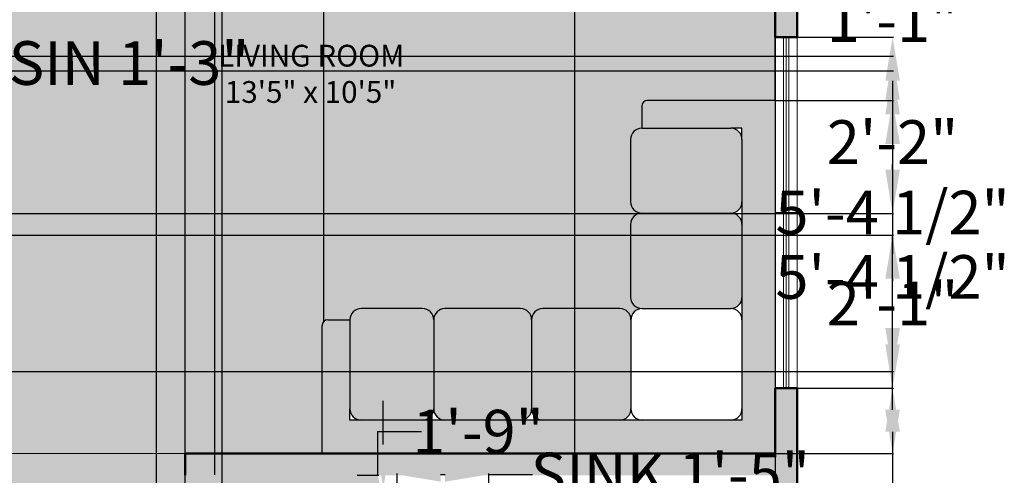
# Model space of a CAD drawing. Units: inches. Extents: x 339 to 824, y 73 to 445.
# Tile 4 of 5: x 605 to 785, y 213 to 297. Entities that reach past the tile are written whole.
import ezdxf

# ---------------------------------------------------------------- set-up
doc = ezdxf.new("R2010")
doc.units = ezdxf.units.IN
doc.header["$MEASUREMENT"] = 0
for name, color, linetype, lineweight in [('A-ANNO-DIMS', 2, 'Continuous', 18), ('A-AREA-IDEN', 7, 'Continuous', 25), ('A-DOOR', 3, 'Continuous', 25), ('A-FLOR-BNDY', 8, 'Continuous', 13), ('A-FLOR-PATT', 8, 'Continuous', 13), ('A-FURN', 9, 'Continuous', 25), ('A-GLAZ', 4, 'Continuous', 18), ('A-WALL', 7, 'Continuous', 50), ('A-WALL-PATT', 1, 'Continuous', 13)]:
    doc.layers.add(name, color=color, linetype=linetype, lineweight=lineweight)
doc.layers.add('A-FURN-PATT', color=251, linetype='Continuous', lineweight=13, true_color=0x6d5f6c)
doc.styles.get("Standard").update_dxf_attribs({"font": 'arial.ttf'})
doc.dimstyles.get("Standard").update_dxf_attribs({"dimtxt": 8, "dimasz": 8, "dimexe": 0.18, "dimexo": 0.0625, "dimgap": 0.09, "dimtad": 0, "dimtih": 1, "dimtoh": 1, "dimdec": 0, "dimzin": 0, "dimdsep": 46, "dimlunit": 3, "dimtxsty": 'Standard', "dimcen": 0.09, "dimadec": 0, "dimazin": 0, "dimtfac": 1, "dimtdec": 0, "dimtofl": 0, "dimtmove": 0, "dimatfit": 3, "dimfxl": 1, "dimtolj": 1, "dimtzin": 0, "dimarcsym": 0})

# ---------------------------------------------------------------- blocks, each defined once
blk = doc.blocks.new('*U3')
for p, q in [((0, 0), (0, 6)), ((40, 0), (40, 6))]:
    blk.add_line(p, q)
blk.add_lwpolyline([(0, 0), (0, -40), (1.75, -40), (1.75, 0)], close=True)
blk.add_arc((0, 0), 40, 270, 0)
blk = doc.blocks.new('*D20')
at = {"layer": 'A-ANNO-DIMS', "color": 0, "lineweight": -2, "transparency": 16777216}
for p, q in [((558.32, 290.78), (558.32, 288.42)), ((573.25, 290.78), (573.25, 288.42)), ((550.32, 288.6), (542.32, 288.6)), ((581.25, 288.6), (589.25, 288.6))]:
    blk.add_line(p, q, dxfattribs=at)
at = {"layer": 'A-ANNO-DIMS', "color": 0, "transparency": 16777216}
for points in [[(550.32, 289.94), (550.32, 287.27), (558.32, 288.6)], [(581.25, 289.94), (581.25, 287.27), (573.25, 288.6)]]:
    blk.add_solid(points, dxfattribs=at)
at = {"layer": 'Defpoints', "color": 0, "transparency": 16777216}
for p in [(558.32, 290.84), (573.25, 290.84), (573.25, 288.6)]:
    blk.add_point(p, dxfattribs=at)
at = {"layer": 'A-ANNO-DIMS', "color": 0, "transparency": 16777216, "insert": (618.12, 288.6), "char_height": 8, "attachment_point": 5}
blk.add_mtext('\\A1;BASIN 1\'-3"', dxfattribs=at)
blk = doc.blocks.new('*D23')
at = {"layer": 'A-ANNO-DIMS', "color": 0, "lineweight": -2, "transparency": 16777216}
for p, q in [((670.64, 213.06), (670.64, 221.06)), ((670.64, 221.06), (678.64, 221.06)), ((666.81, 213.06), (670.82, 213.06)), ((670.64, 200.11), (670.64, 205.06)), ((666.81, 192.11), (670.82, 192.11))]:
    blk.add_line(p, q, dxfattribs=at)
at = {"layer": 'A-ANNO-DIMS', "color": 0, "transparency": 16777216}
for points in [[(669.31, 205.06), (671.98, 205.06), (670.64, 213.06)], [(669.31, 200.11), (671.98, 200.11), (670.64, 192.11)]]:
    blk.add_solid(points, dxfattribs=at)
at = {"layer": 'Defpoints', "color": 0, "transparency": 16777216}
for p in [(666.74, 213.06), (670.64, 213.06), (666.74, 192.11)]:
    blk.add_point(p, dxfattribs=at)
at = {"layer": 'A-ANNO-DIMS', "color": 0, "transparency": 16777216, "insert": (688.99, 221.06), "char_height": 8, "attachment_point": 5}
blk.add_mtext('\\A1;1\'-9"', dxfattribs=at)
blk = doc.blocks.new('*D24')
at = {"layer": 'A-ANNO-DIMS', "color": 0, "lineweight": -2, "transparency": 16777216}
for p, q in [((674.13, 210.76), (674.13, 213.4)), ((682.13, 213.22), (682.94, 213.22)), ((690.94, 210.76), (690.94, 213.4)), ((690.94, 213.22), (698.94, 213.22))]:
    blk.add_line(p, q, dxfattribs=at)
at = {"layer": 'A-ANNO-DIMS', "color": 0, "transparency": 16777216}
for points in [[(682.13, 214.56), (682.13, 211.89), (674.13, 213.22)], [(682.94, 214.56), (682.94, 211.89), (690.94, 213.22)]]:
    blk.add_solid(points, dxfattribs=at)
at = {"layer": 'Defpoints', "color": 0, "transparency": 16777216}
for p in [(690.94, 213.22), (674.13, 210.7), (690.94, 210.7)]:
    blk.add_point(p, dxfattribs=at)
at = {"layer": 'A-ANNO-DIMS', "color": 0, "transparency": 16777216, "insert": (724.24, 213.22), "char_height": 8, "attachment_point": 5}
blk.add_mtext('\\A1;SINK 1\'-5"', dxfattribs=at)
blk = doc.blocks.new('*D25')
at = {"layer": 'A-ANNO-DIMS', "color": 0, "lineweight": -2, "transparency": 16777216}
for p, q in [((671.61, 218.7), (671.61, 226.7)), ((674.07, 210.7), (671.43, 210.7)), ((674.07, 199.5), (671.43, 199.5)), ((671.61, 191.5), (671.61, 183.5))]:
    blk.add_line(p, q, dxfattribs=at)
at = {"layer": 'A-ANNO-DIMS', "color": 0, "transparency": 16777216}
for points in [[(670.28, 218.7), (672.95, 218.7), (671.61, 210.7)], [(670.28, 191.5), (672.95, 191.5), (671.61, 199.5)]]:
    blk.add_solid(points, dxfattribs=at)
at = {"layer": 'Defpoints', "color": 0, "transparency": 16777216}
for p in [(671.61, 210.7), (674.13, 210.7), (674.13, 199.5)]:
    blk.add_point(p, dxfattribs=at)
at = {"layer": 'A-ANNO-DIMS', "color": 0, "transparency": 16777216, "insert": (671.61, 205.1), "char_height": 8, "attachment_point": 5}
blk.add_mtext('\\A1;0\'-11"', dxfattribs=at)
blk = doc.blocks.new('*D36')
at = {"layer": 'A-ANNO-DIMS', "color": 0, "lineweight": -2, "transparency": 16777216}
for p, q in [((747.55, 229.04), (765.16, 229.04)), ((764.98, 221.04), (764.98, 169.72)), ((764.98, 110.06), (764.98, 161.37)), ((747.55, 102.06), (765.16, 102.06))]:
    blk.add_line(p, q, dxfattribs=at)
at = {"layer": 'A-ANNO-DIMS', "color": 0, "transparency": 16777216}
for points in [[(763.65, 221.04), (766.32, 221.04), (764.98, 229.04)], [(763.65, 110.06), (766.32, 110.06), (764.98, 102.06)]]:
    blk.add_solid(points, dxfattribs=at)
at = {"layer": 'Defpoints', "color": 0, "transparency": 16777216}
for p in [(747.48, 229.04), (764.98, 229.04), (747.48, 102.06)]:
    blk.add_point(p, dxfattribs=at)
at = {"layer": 'A-ANNO-DIMS', "color": 0, "transparency": 16777216, "insert": (764.98, 165.55), "char_height": 8, "attachment_point": 5}
blk.add_mtext('\\A1;10\'-7"', dxfattribs=at)
blk = doc.blocks.new('*D37')
at = {"layer": 'A-ANNO-DIMS', "color": 0, "lineweight": -2, "transparency": 16777216}
for p, q in [((747.55, 293.36), (765.16, 293.36)), ((764.98, 285.36), (764.98, 265.43)), ((764.98, 237.04), (764.98, 256.97)), ((747.55, 229.04), (765.16, 229.04))]:
    blk.add_line(p, q, dxfattribs=at)
at = {"layer": 'A-ANNO-DIMS', "color": 0, "transparency": 16777216}
for points in [[(763.65, 285.36), (766.32, 285.36), (764.98, 293.36)], [(763.65, 237.04), (766.32, 237.04), (764.98, 229.04)]]:
    blk.add_solid(points, dxfattribs=at)
at = {"layer": 'Defpoints', "color": 0, "transparency": 16777216}
for p in [(747.48, 293.36), (764.98, 293.36), (747.48, 229.04)]:
    blk.add_point(p, dxfattribs=at)
at = {"layer": 'A-ANNO-DIMS', "color": 0, "transparency": 16777216, "insert": (764.98, 261.2), "char_height": 8, "attachment_point": 5}
blk.add_mtext('\\A1;5\'-4 1/2"', dxfattribs=at)
blk = doc.blocks.new('*D38')
at = {"layer": 'A-ANNO-DIMS', "color": 0, "lineweight": -2, "transparency": 16777216}
for p, q in [((592.11, 433.56), (584.11, 433.56)), ((600.11, 213.12), (600.11, 433.74)), ((635.29, 213.12), (635.29, 433.74)), ((643.29, 433.56), (651.29, 433.56))]:
    blk.add_line(p, q, dxfattribs=at)
at = {"layer": 'A-ANNO-DIMS', "color": 0, "transparency": 16777216}
for points in [[(592.11, 434.89), (592.11, 432.23), (600.11, 433.56)], [(643.29, 434.89), (643.29, 432.23), (635.29, 433.56)]]:
    blk.add_solid(points, dxfattribs=at)
at = {"layer": 'Defpoints', "color": 0, "transparency": 16777216}
for p in [(635.29, 433.56), (600.11, 213.06), (635.29, 213.06)]:
    blk.add_point(p, dxfattribs=at)
at = {"layer": 'A-ANNO-DIMS', "color": 0, "transparency": 16777216, "insert": (617.7, 433.56), "char_height": 8, "attachment_point": 5}
blk.add_mtext('\\A1;2\'-11"', dxfattribs=at)
blk = doc.blocks.new('*D39')
at = {"layer": 'A-ANNO-DIMS', "color": 0, "lineweight": -2, "transparency": 16777216}
for p, q in [((706.66, 342), (706.66, 84.38)), ((743.48, 342), (743.48, 84.38)), ((698.66, 84.56), (690.66, 84.56)), ((751.48, 84.56), (759.48, 84.56))]:
    blk.add_line(p, q, dxfattribs=at)
at = {"layer": 'A-ANNO-DIMS', "color": 0, "transparency": 16777216}
for points in [[(698.66, 85.89), (698.66, 83.23), (706.66, 84.56)], [(751.48, 85.89), (751.48, 83.23), (743.48, 84.56)]]:
    blk.add_solid(points, dxfattribs=at)
at = {"layer": 'Defpoints', "color": 0, "transparency": 16777216}
for p in [(706.66, 342.06), (743.48, 342.06), (743.48, 84.56)]:
    blk.add_point(p, dxfattribs=at)
at = {"layer": 'A-ANNO-DIMS', "color": 0, "transparency": 16777216, "insert": (725.07, 84.56), "char_height": 8, "attachment_point": 5}
blk.add_mtext('\\A1;3\'-1"', dxfattribs=at)
blk = doc.blocks.new('*D42')
at = {"layer": 'A-ANNO-DIMS', "color": 0, "lineweight": -2, "transparency": 16777216}
for p, q in [((582.55, 257.06), (765.16, 257.06)), ((764.98, 249.06), (764.98, 248.67)), ((764.98, 240.06), (764.98, 240.45)), ((582.55, 232.06), (765.16, 232.06))]:
    blk.add_line(p, q, dxfattribs=at)
at = {"layer": 'A-ANNO-DIMS', "color": 0, "transparency": 16777216}
for points in [[(763.65, 249.06), (766.32, 249.06), (764.98, 257.06)], [(763.65, 240.06), (766.32, 240.06), (764.98, 232.06)]]:
    blk.add_solid(points, dxfattribs=at)
at = {"layer": 'Defpoints', "color": 0, "transparency": 16777216}
for p in [(582.48, 257.06), (582.48, 232.06), (764.98, 232.06)]:
    blk.add_point(p, dxfattribs=at)
at = {"layer": 'A-ANNO-DIMS', "color": 0, "transparency": 16777216, "insert": (764.98, 244.56), "char_height": 8, "attachment_point": 5}
blk.add_mtext('\\A1;2\'-1"', dxfattribs=at)
blk = doc.blocks.new('*D44')
at = {"layer": 'A-ANNO-DIMS', "color": 0, "lineweight": -2, "transparency": 16777216}
for p, q in [((553.55, 287.19), (765.16, 287.19)), ((764.98, 279.19), (764.98, 278.23)), ((764.98, 269.06), (764.98, 270.02)), ((553.55, 261.06), (765.16, 261.06))]:
    blk.add_line(p, q, dxfattribs=at)
at = {"layer": 'A-ANNO-DIMS', "color": 0, "transparency": 16777216}
for points in [[(763.65, 279.19), (766.32, 279.19), (764.98, 287.19)], [(763.65, 269.06), (766.32, 269.06), (764.98, 261.06)]]:
    blk.add_solid(points, dxfattribs=at)
at = {"layer": 'Defpoints', "color": 0, "transparency": 16777216}
for p in [(553.48, 287.19), (764.98, 287.19), (553.48, 261.06)]:
    blk.add_point(p, dxfattribs=at)
at = {"layer": 'A-ANNO-DIMS', "color": 0, "transparency": 16777216, "insert": (764.98, 274.12), "char_height": 8, "attachment_point": 5}
blk.add_mtext('\\A1;2\'-2"', dxfattribs=at)
blk = doc.blocks.new('*D46')
at = {"layer": 'A-ANNO-DIMS', "color": 0, "lineweight": -2, "transparency": 16777216}
for p, q in [((764.98, 311.06), (764.98, 319.06)), ((578.55, 303.06), (765.16, 303.06)), ((578.55, 289.86), (765.16, 289.86)), ((764.98, 281.86), (764.98, 273.86))]:
    blk.add_line(p, q, dxfattribs=at)
at = {"layer": 'A-ANNO-DIMS', "color": 0, "transparency": 16777216}
for points in [[(763.65, 311.06), (766.32, 311.06), (764.98, 303.06)], [(763.65, 281.86), (766.32, 281.86), (764.98, 289.86)]]:
    blk.add_solid(points, dxfattribs=at)
at = {"layer": 'Defpoints', "color": 0, "transparency": 16777216}
for p in [(578.48, 303.06), (578.48, 289.86), (764.98, 289.86)]:
    blk.add_point(p, dxfattribs=at)
at = {"layer": 'A-ANNO-DIMS', "color": 0, "transparency": 16777216, "insert": (764.98, 296.46), "char_height": 8, "attachment_point": 5}
blk.add_mtext('\\A1;1\'-1"', dxfattribs=at)
blk = doc.blocks.new('*D53')
at = {"layer": 'A-ANNO-DIMS', "color": 0, "lineweight": -2, "transparency": 16777216}
for p, q in [((630, 375), (630, 84.38)), ((642, 375), (642, 84.38)), ((622, 84.56), (614, 84.56)), ((650, 84.56), (658, 84.56))]:
    blk.add_line(p, q, dxfattribs=at)
at = {"layer": 'A-ANNO-DIMS', "color": 0, "transparency": 16777216}
for points in [[(622, 85.89), (622, 83.23), (630, 84.56)], [(650, 85.89), (650, 83.23), (642, 84.56)]]:
    blk.add_solid(points, dxfattribs=at)
at = {"layer": 'Defpoints', "color": 0, "transparency": 16777216}
for p in [(630, 375.06), (642, 375.06), (642, 84.56)]:
    blk.add_point(p, dxfattribs=at)
at = {"layer": 'A-ANNO-DIMS', "color": 0, "transparency": 16777216, "insert": (668.35, 84.56), "char_height": 8, "attachment_point": 5}
blk.add_mtext('\\A1;1\'-0"', dxfattribs=at)
blk = doc.blocks.new('*D55')
at = {"layer": 'A-ANNO-DIMS', "color": 0, "lineweight": -2, "transparency": 16777216}
for p, q in [((582.48, 213.12), (582.48, 433.74)), ((590.48, 433.56), (592.11, 433.56)), ((600.11, 213.12), (600.11, 433.74)), ((600.11, 433.56), (608.11, 433.56))]:
    blk.add_line(p, q, dxfattribs=at)
at = {"layer": 'A-ANNO-DIMS', "color": 0, "transparency": 16777216}
for points in [[(590.48, 434.89), (590.48, 432.23), (582.48, 433.56)], [(592.11, 434.89), (592.11, 432.23), (600.11, 433.56)]]:
    blk.add_solid(points, dxfattribs=at)
at = {"layer": 'Defpoints', "color": 0, "transparency": 16777216}
for p in [(600.11, 433.56), (582.48, 213.06), (600.11, 213.06)]:
    blk.add_point(p, dxfattribs=at)
at = {"layer": 'A-ANNO-DIMS', "color": 0, "transparency": 16777216, "insert": (627.78, 433.56), "char_height": 8, "attachment_point": 5}
blk.add_mtext('\\A1;1\'-5 1/2"', dxfattribs=at)
blk = doc.blocks.new('*D57')
at = {"layer": 'A-ANNO-DIMS', "color": 0, "lineweight": -2, "transparency": 16777216}
for p, q in [((660.7, 241.32), (660.7, 433.74)), ((668.7, 433.56), (688.24, 433.56)), ((735.48, 433.56), (715.95, 433.56)), ((743.48, 281.81), (743.48, 433.74))]:
    blk.add_line(p, q, dxfattribs=at)
at = {"layer": 'A-ANNO-DIMS', "color": 0, "transparency": 16777216}
for points in [[(668.7, 434.89), (668.7, 432.23), (660.7, 433.56)], [(735.48, 434.89), (735.48, 432.23), (743.48, 433.56)]]:
    blk.add_solid(points, dxfattribs=at)
at = {"layer": 'Defpoints', "color": 0, "transparency": 16777216}
for p in [(743.48, 433.56), (743.48, 281.75), (660.7, 241.26)]:
    blk.add_point(p, dxfattribs=at)
at = {"layer": 'A-ANNO-DIMS', "color": 0, "transparency": 16777216, "insert": (702.09, 433.56), "char_height": 8, "attachment_point": 5}
blk.add_mtext('\\A1;6\'-11"', dxfattribs=at)
blk = doc.blocks.new('*D58')
at = {"layer": 'A-ANNO-DIMS', "color": 0, "lineweight": -2, "transparency": 16777216}
for p, q in [((743.55, 281.75), (765.16, 281.75)), ((764.98, 273.75), (764.98, 253.63)), ((764.98, 225.06), (764.98, 245.18)), ((743.55, 217.06), (765.16, 217.06))]:
    blk.add_line(p, q, dxfattribs=at)
at = {"layer": 'A-ANNO-DIMS', "color": 0, "transparency": 16777216}
for points in [[(763.65, 273.75), (766.32, 273.75), (764.98, 281.75)], [(763.65, 225.06), (766.32, 225.06), (764.98, 217.06)]]:
    blk.add_solid(points, dxfattribs=at)
at = {"layer": 'Defpoints', "color": 0, "transparency": 16777216}
for p in [(743.48, 281.75), (764.98, 281.75), (743.48, 217.06)]:
    blk.add_point(p, dxfattribs=at)
at = {"layer": 'A-ANNO-DIMS', "color": 0, "transparency": 16777216, "insert": (764.98, 249.4), "char_height": 8, "attachment_point": 5}
blk.add_mtext('\\A1;5\'-4 1/2"', dxfattribs=at)
blk = doc.blocks.new('*D63')
at = {"layer": 'A-ANNO-DIMS', "color": 0, "lineweight": -2, "transparency": 16777216}
for p, q in [((627.29, 433.56), (619.29, 433.56)), ((635.29, 213.12), (635.29, 433.74)), ((640.73, 213.12), (640.73, 433.74)), ((648.73, 433.56), (656.73, 433.56))]:
    blk.add_line(p, q, dxfattribs=at)
at = {"layer": 'A-ANNO-DIMS', "color": 0, "transparency": 16777216}
for points in [[(627.29, 434.89), (627.29, 432.23), (635.29, 433.56)], [(648.73, 434.89), (648.73, 432.23), (640.73, 433.56)]]:
    blk.add_solid(points, dxfattribs=at)
at = {"layer": 'Defpoints', "color": 0, "transparency": 16777216}
for p in [(640.73, 433.56), (635.29, 213.06), (640.73, 213.06)]:
    blk.add_point(p, dxfattribs=at)
at = {"layer": 'A-ANNO-DIMS', "color": 0, "transparency": 16777216, "insert": (676.77, 433.56), "char_height": 8, "attachment_point": 5}
blk.add_mtext('\\A1;0\'-5 1/2"', dxfattribs=at)

msp = doc.modelspace()

# ---------------------------------------------------------------- hatches: boundary and pattern name
at = {"layer": 'A-FLOR-PATT'}
h = msp.add_hatch(color=256, dxfattribs=at)
h.dxf.hatch_style = 1
h.paths.add_polyline_path([(661.42, 241.56), (665.51, 241.56, -0.414214), (667.55, 243.6), (678.83, 243.6, -0.414214), (680.87, 241.56, -0.414214), (682.91, 243.6), (696.76, 243.6, -0.414214), (698.8, 241.56, -0.414214), (700.84, 243.6), (714.97, 243.6, -0.412935), (717.02, 241.56, -0.410727), (719.02, 243.61, -0.419077), (716.95, 245.66), (716.95, 259.06, -0.414214), (718.99, 261.11, -0.414214), (716.95, 263.15), (716.95, 274.6, -0.414214), (718.99, 276.64), (718.99, 280.73, -0.414214), (720.01, 281.75), (743.48, 281.75), (743.48, 293.36), (743.48, 299.72), (741.87, 299.72), (741.87, 299.75, -0.401453), (706.66, 336.54), (706.66, 342.06), (582.48, 342.06), (582.48, 307.06), (582.48, 217.06), (635.29, 217.06), (660.4, 217.06), (660.4, 240.53, -0.414214)])
h.paths.add_polyline_path([(639.94, 279.04), (679.09, 279.04), (679.09, 293.92), (639.94, 293.92)], flags=24)
h = msp.add_hatch(color=256, dxfattribs=at)
h.dxf.hatch_style = 1
h.paths.add_polyline_path([(578.48, 106.06), (710.48, 106.06), (710.48, 130.47), (706.48, 130.47), (706.48, 137.8), (692.06, 137.8), (692.06, 195.19), (670.62, 195.11), (670.62, 213.06), (635.29, 213.06), (635.29, 217.06), (600.11, 217.06), (600.11, 213.06), (582.48, 213.06), (582.48, 147.67), (578.48, 147.67)])
h.paths.add_polyline_path([(600.11, 174.62), (600.11, 209.78), (601.65, 209.78), (601.65, 174.62)], flags=16)
h.paths.add_polyline_path([(630.19, 155.1), (658.99, 155.1), (658.99, 168.27), (630.19, 168.27)], flags=24)
h = msp.add_hatch(color=256, dxfattribs=at)
h.dxf.hatch_style = 1
h.paths.add_polyline_path([(710.48, 106.06), (710.48, 130.47), (706.48, 130.47), (706.48, 137.8), (692.06, 137.8), (692.06, 195.19), (670.62, 195.11), (670.62, 213.06), (635.29, 213.06), (635.29, 217.06), (600.11, 217.06), (600.11, 213.06), (582.48, 213.06), (582.48, 147.67), (582.91, 106.06)])
h.paths.add_polyline_path([(601.65, 174.62), (600.11, 174.62), (600.11, 209.78), (601.65, 209.78)], flags=16)
h.paths.add_polyline_path([(630.19, 155.1), (658.99, 155.1), (658.99, 168.27), (630.19, 168.27)], flags=24)
at = {"layer": 'A-FURN-PATT'}
h = msp.add_hatch(color=256, dxfattribs=at)
h.dxf.hatch_style = 1
h.paths.add_polyline_path([(743.48, 217.06), (743.48, 281.75), (720.01, 281.75, 0.414214), (718.99, 280.73), (718.99, 276.64), (735.32, 276.64), (737.36, 276.64), (737.36, 274.6), (737.36, 225.23), (737.36, 223.18), (735.32, 223.18), (678.83, 223.18), (667.55, 223.18), (665.51, 223.18), (665.51, 225.23), (665.51, 241.56), (661.42, 241.56, 0.414214), (660.4, 240.53), (660.4, 217.06)])
h = msp.add_hatch(color=256, dxfattribs=at)
h.dxf.hatch_style = 1
h.paths.add_polyline_path([(743.48, 217.06), (743.48, 281.75), (720.01, 281.75, 0.414214), (718.99, 280.73), (718.99, 276.64), (735.32, 276.64), (737.36, 276.64), (737.36, 274.6), (737.36, 225.23), (737.36, 223.18), (735.32, 223.18), (678.83, 223.18), (667.55, 223.18), (665.51, 223.18), (665.51, 225.23), (665.51, 241.56), (661.42, 241.56, 0.414214), (660.4, 240.53), (660.4, 217.06)])
h = msp.add_hatch(color=256, dxfattribs=at)
h.dxf.hatch_style = 1
h.paths.add_polyline_path([(660.4, 217.06), (743.48, 217.06), (743.48, 281.75), (720.01, 281.75, 0.414214), (718.99, 280.73), (718.99, 276.64), (735.32, 276.64), (737.36, 276.64), (737.36, 274.6), (737.36, 225.23), (737.36, 223.18), (735.32, 223.18), (678.83, 223.18), (667.55, 223.18), (665.51, 223.18), (665.51, 225.23), (665.51, 241.56), (661.42, 241.56, 0.414214), (660.4, 240.53)])
h = msp.add_hatch(color=256, dxfattribs=at)
h.dxf.hatch_style = 1
h.paths.add_polyline_path([(665.51, 225.23), (665.51, 241.56), (661.42, 241.56, 0.414214), (660.4, 240.53), (660.4, 217.06), (743.48, 217.06), (743.48, 281.75), (720.01, 281.75, 0.414214), (718.99, 280.73), (718.99, 276.64), (735.32, 276.64), (737.36, 276.64), (737.36, 274.6), (737.36, 225.23), (737.36, 223.18), (735.32, 223.18), (678.83, 223.18), (667.55, 223.18), (665.51, 223.18)])
h = msp.add_hatch(color=256, dxfattribs=at)
h.dxf.hatch_style = 1
h.paths.add_polyline_path([(678.83, 223.18), (667.55, 223.18), (665.51, 223.18), (665.51, 225.23), (665.51, 241.56), (661.42, 241.56, 0.414214), (660.4, 240.53), (660.4, 217.06), (743.48, 217.06), (743.48, 281.75), (720.01, 281.75, 0.414214), (718.99, 280.73), (718.99, 276.64), (735.32, 276.64), (737.36, 276.64), (737.36, 274.6), (737.36, 225.23), (737.36, 223.18), (735.32, 223.18)])
h = msp.add_hatch(color=256, dxfattribs=at)
h.dxf.hatch_style = 1
h.paths.add_polyline_path([(735.32, 261.11, 0.414214), (737.36, 263.15), (737.36, 274.6, 0.414214), (735.32, 276.64), (718.99, 276.64, 0.414214), (716.95, 274.6), (716.95, 263.15, 0.414214), (718.99, 261.11)])
h = msp.add_hatch(color=256, dxfattribs=at)
h.dxf.hatch_style = 1
h.paths.add_polyline_path([(735.32, 243.61, 0.414214), (737.36, 245.66), (737.36, 259.06, 0.414214), (735.32, 261.11), (718.99, 261.11, 0.414214), (716.95, 259.06), (716.95, 245.66, 0.414214), (718.99, 243.61)])
h = msp.add_hatch(color=256, dxfattribs=at)
h.dxf.hatch_style = 1
h.paths.add_polyline_path([(680.87, 241.56, 0.414214), (678.83, 243.6), (667.55, 243.6, 0.414214), (665.51, 241.56), (665.51, 225.23, 0.414214), (667.55, 223.18), (678.83, 223.18, 0.414214), (680.87, 225.23)])
h = msp.add_hatch(color=256, dxfattribs=at)
h.dxf.hatch_style = 1
h.paths.add_polyline_path([(696.76, 223.18, 0.414214), (698.8, 225.23), (698.8, 241.56, 0.414214), (696.76, 243.6), (682.91, 243.6, 0.414214), (680.87, 241.56), (680.87, 225.23, 0.414214), (682.91, 223.18)])
h = msp.add_hatch(color=256, dxfattribs=at)
h.dxf.hatch_style = 1
h.paths.add_polyline_path([(700.84, 243.6, 0.414214), (698.8, 241.56), (698.8, 225.23, 0.414214), (700.84, 223.18), (714.97, 223.18, 0.414214), (717.02, 225.23), (717.02, 241.56, 0.414214), (714.97, 243.6)])
at = {"layer": 'A-WALL-PATT'}
h = msp.add_hatch(color=256, dxfattribs=at)
h.dxf.hatch_style = 1
h.paths.add_polyline_path([(747.48, 416.06), (743.48, 416.06), (743.48, 293.36), (747.48, 293.36)])
h = msp.add_hatch(color=256, dxfattribs=at)
h.dxf.hatch_style = 1
h.paths.add_polyline_path([(675.71, 106.06), (675.71, 102.06), (743.48, 102.06), (747.48, 102.06), (747.48, 229.04), (743.48, 229.04), (743.48, 217.06), (660.4, 217.06), (635.29, 217.06), (635.29, 213.06), (743.48, 213.06), (743.48, 106.06)])

# ---------------------------------------------------------------- linework, layer by layer
at = {"layer": 'A-FLOR-BNDY'}
msp.add_line((582.48, 217.06), (635.29, 217.06), dxfattribs=at)
at = {"layer": 'A-FURN'}
for p, q in [((743.48, 281.75), (720.01, 281.75)), ((743.48, 281.75), (743.48, 217.06)), ((718.99, 280.73), (718.99, 276.64)), ((718.99, 276.64), (735.32, 276.64)), ((718.99, 276.64), (718.99, 276.64)), ((737.36, 276.64), (735.32, 276.64)), ((737.36, 274.6), (737.36, 276.64)), ((716.95, 274.6), (716.95, 263.15)), ((737.36, 274.6), (737.36, 223.18)), ((718.99, 261.11), (735.32, 261.11)), ((716.95, 259.06), (716.95, 245.66)), ((678.83, 243.6), (667.55, 243.6)), ((696.76, 243.6), (682.91, 243.6)), ((714.97, 243.6), (700.84, 243.6)), ((718.99, 243.61), (735.32, 243.61)), ((660.4, 217.06), (660.4, 240.53)), ((661.42, 241.56), (665.51, 241.56)), ((665.51, 241.56), (665.51, 225.23)), ((665.51, 241.56), (665.51, 241.56)), ((680.87, 241.56), (680.87, 225.23)), ((698.8, 241.56), (698.8, 225.23)), ((717.02, 241.57), (717.02, 225.23)), ((665.51, 223.18), (665.51, 225.23)), ((737.36, 225.23), (737.36, 223.18)), ((667.55, 223.18), (665.51, 223.18)), ((678.83, 223.18), (667.55, 223.18)), ((737.36, 223.18), (678.83, 223.18)), ((737.36, 223.18), (735.32, 223.18)), ((743.48, 217.06), (660.4, 217.06))]:
    msp.add_line(p, q, dxfattribs=at)
for centre, radius, start, end in [((720.01, 280.73), 1.02, 90, 180), ((718.99, 274.6), 2.04, 90, 180), ((735.32, 274.6), 2.04, 0, 90), ((718.99, 263.15), 2.04, 180, 270), ((735.32, 263.15), 2.04, 270, 0), ((718.99, 259.06), 2.04, 90, 90), ((718.99, 259.06), 2.04, 90, 180), ((735.32, 259.06), 2.04, 0, 90), ((718.99, 245.66), 2.04, 180, 270), ((735.32, 245.66), 2.04, 270, 0), ((667.55, 241.56), 2.04, 90, 180), ((678.83, 241.56), 2.04, 0, 90), ((682.91, 241.56), 2.04, 90, 180), ((696.76, 241.56), 2.04, 0, 0), ((696.76, 241.56), 2.04, 0, 90), ((700.84, 241.56), 2.04, 90, 180), ((714.97, 241.56), 2.04, 0, 90), ((719.06, 241.57), 2.04, 90, 180), ((735.32, 241.57), 2.04, 0, 90), ((661.42, 240.53), 1.02, 90, 180), ((667.55, 225.23), 2.04, 180, 270), ((678.83, 225.23), 2.04, 270, 0), ((682.91, 225.23), 2.04, 180, 270), ((696.76, 225.23), 2.04, 270, 0), ((700.84, 225.23), 2.04, 180, 270), ((714.97, 225.23), 2.04, 270, 0), ((719.06, 225.23), 2.04, 180, 270), ((735.32, 225.23), 2.04, 270, 0)]:
    msp.add_arc(centre, radius, start, end, dxfattribs=at)
at = {"layer": 'A-GLAZ'}
for p, q in [((743.48, 293.36), (743.48, 229.04)), ((744.98, 293.36), (744.98, 229.04)), ((745.48, 293.36), (745.48, 229.04)), ((745.98, 293.36), (745.98, 229.04)), ((747.48, 293.36), (747.48, 229.04)), ((743.48, 261.2), (747.48, 261.2)), ((747.48, 229.04), (743.48, 229.04))]:
    msp.add_line(p, q, dxfattribs=at)
at = {"layer": 'A-WALL'}
for p, q in [((743.48, 293.36), (743.48, 416.06)), ((747.48, 416.06), (747.48, 293.36)), ((743.48, 293.36), (747.48, 293.36)), ((743.48, 229.04), (747.48, 229.04)), ((743.48, 217.06), (743.48, 229.04)), ((747.48, 229.04), (747.48, 102.06)), ((635.29, 213.06), (635.29, 217.06)), ((635.29, 217.06), (743.48, 217.06))]:
    msp.add_line(p, q, dxfattribs=at)

# ---------------------------------------------------------------- block references
at = {"layer": 'A-DOOR', "xscale": 0.8792070118950395, "yscale": 0.8792070118950395, "zscale": 0.8792070118950395}
msp.add_blockref('*U3', (600.11, 209.78), dxfattribs=at)

# ---------------------------------------------------------------- texts
at = {"layer": 'A-AREA-IDEN', "insert": (641.34, 291.94), "char_height": 3.9887, "attachment_point": 1}
msp.add_mtext_dynamic_manual_height_columns('LIVING ROOM\\P 13\'5" x 10\'5"', width=44.4226, gutter_width=19.94, heights=[0], dxfattribs=at)

# ---------------------------------------------------------------- dimensions: what is measured, and where the dimension line sits
at = {"layer": 'A-ANNO-DIMS'}
for base, p1, p2, picture, middle in [((600.11, 433.56), (582.48, 213.06), (600.11, 213.06), '*D55', (627.78, 433.56)), ((640.73, 433.56), (635.29, 213.06), (640.73, 213.06), '*D63', (676.77, 433.56)), ((635.29, 433.56), (600.11, 213.06), (635.29, 213.06), '*D38', (617.7, 433.56)), ((743.48, 433.56), (660.7, 241.26), (743.48, 281.75), '*D57', (702.09, 433.56)), ((642, 84.56), (630, 375.06), (642, 375.06), '*D53', (668.35, 84.56)), ((743.48, 84.56), (706.66, 342.06), (743.48, 342.06), '*D39', (725.07, 84.56))]:
    dim = msp.add_linear_dim(base=base, p1=p1, p2=p2, dimstyle='Standard', override={"dimdec": 1, "dimlfac": 1, "dimrnd": 0, "dimzin": 1, "dimdsep": 46, "dimlunit": 4, "dimfrac": 2}, dxfattribs=at)
    dim.commit()
    dim.dimension.update_dxf_attribs({"geometry": picture, "text_midpoint": middle})
for base, p1, p2, picture, middle in [((764.98, 289.86), (578.48, 303.06), (578.48, 289.86), '*D46', (764.98, 296.46)), ((764.98, 293.36), (747.48, 229.04), (747.48, 293.36), '*D37', (764.98, 261.2)), ((764.98, 287.19), (553.48, 261.06), (553.48, 287.19), '*D44', (764.98, 274.12)), ((764.98, 281.75), (743.48, 217.06), (743.48, 281.75), '*D58', (764.98, 249.4)), ((764.98, 232.06), (582.48, 257.06), (582.48, 232.06), '*D42', (764.98, 244.56)), ((764.98, 229.04), (747.48, 102.06), (747.48, 229.04), '*D36', (764.98, 165.55)), ((671.61, 210.7), (674.13, 199.5), (674.13, 210.7), '*D25', (671.61, 205.1)), ((670.6446, 213.0602), (666.7427, 192.1052), (666.7427, 213.0602), '*D23', (688.9911, 221.0602))]:
    dim = msp.add_linear_dim(base=base, p1=p1, p2=p2, angle=90, dimstyle='Standard', override={"dimdec": 1, "dimlfac": 1, "dimrnd": 0, "dimzin": 1, "dimdsep": 46, "dimlunit": 4, "dimfrac": 2}, dxfattribs=at)
    dim.commit()
    dim.dimension.update_dxf_attribs({"geometry": picture, "text_midpoint": middle})
for base, p1, p2, text, picture, middle in [((573.25, 288.6), (558.32, 290.84), (573.25, 290.84), 'BASIN <>', '*D20', (618.12, 288.6)), ((690.94, 213.22), (674.13, 210.7), (690.94, 210.7), 'SINK <>', '*D24', (724.24, 213.22))]:
    dim = msp.add_linear_dim(base=base, p1=p1, p2=p2, text=text, dimstyle='Standard', override={"dimdec": 1, "dimlfac": 1, "dimrnd": 0, "dimzin": 1, "dimdsep": 46, "dimlunit": 4, "dimfrac": 2}, dxfattribs=at)
    dim.commit()
    dim.dimension.update_dxf_attribs({"geometry": picture, "text_midpoint": middle})

doc.saveas('drawing.dxf')
